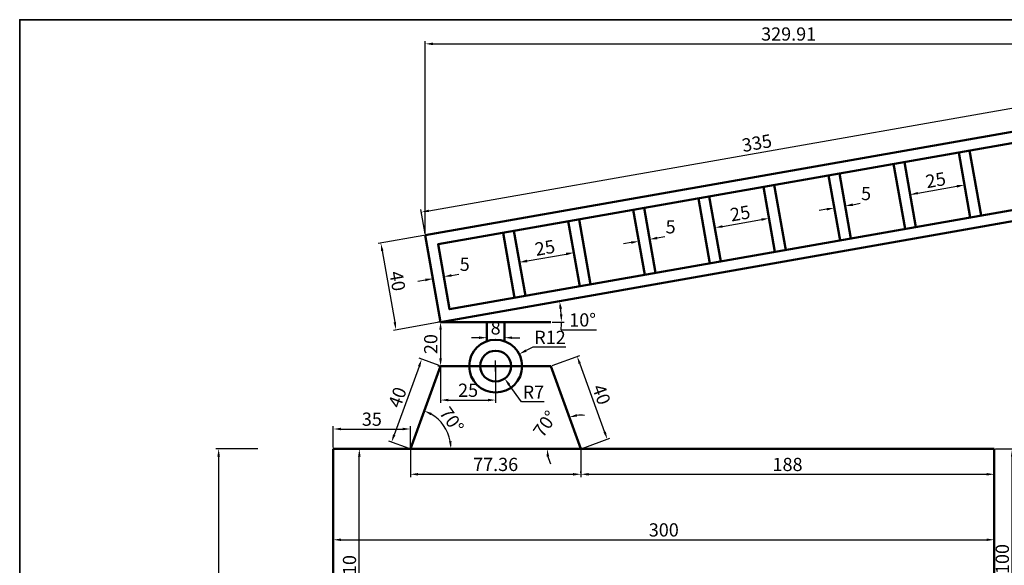
# Model space of a CAD drawing. Units: millimetres. Extents: x -71 to 780, y -41 to 454.
# Tile 2 of 4: x -71 to 376, y 206 to 454. Entities that reach past the tile are written whole.
import ezdxf

# ---------------------------------------------------------------- set-up
doc = ezdxf.new("R2010")
doc.units = ezdxf.units.MM
for name, color, linetype, lineweight in [('M-DIMS', 2, 'Continuous', 25), ('M-OUTL', 7, 'Continuous', 50), ('M-TTLB', 7, 'Continuous', 35)]:
    doc.layers.add(name, color=color, linetype=linetype, lineweight=lineweight)
doc.styles.get("Standard").update_dxf_attribs({"font": 'arial.ttf'})
doc.dimstyles.new('ISO-25', dxfattribs={"dimtxt": 6, "dimasz": 3.5, "dimexe": 1.25, "dimexo": 0.625, "dimtad": 1, "dimtoh": 1, "dimdec": 0, "dimtxsty": 'Standard', "dimcen": 2.5, "dimadec": 0, "dimazin": 0, "dimtfac": 1, "dimtdec": 0, "dimtofl": 0, "dimtmove": 0, "dimatfit": 3, "dimfxl": 1, "dimarcsym": 0})

# ---------------------------------------------------------------- blocks, each defined once
blk = doc.blocks.new('*D10')
at = {"layer": 'Defpoints', "color": 0, "transparency": 16777216}
for p in [(37.81, 259.32), (19.33, 119.32), (37.81, 119.32)]:
    blk.add_point(p, dxfattribs=at)
at = {"layer": 'M-DIMS', "color": 0, "lineweight": -2, "transparency": 16777216}
for p, q in [((37.19, 259.32), (18.08, 259.32)), ((19.33, 255.82), (19.33, 122.82)), ((37.19, 119.32), (18.08, 119.32))]:
    blk.add_line(p, q, dxfattribs=at)
at = {"layer": 'M-DIMS', "color": 0, "transparency": 16777216}
for points in [[(18.74, 255.82), (19.91, 255.82), (19.33, 259.32)], [(18.74, 122.82), (19.91, 122.82), (19.33, 119.32)]]:
    blk.add_solid(points, dxfattribs=at)
at = {"layer": 'M-DIMS', "color": 0, "transparency": 16777216, "insert": (15.64, 189.32), "char_height": 6, "attachment_point": 5, "rotation": 90}
blk.add_mtext('140', dxfattribs=at)
blk = doc.blocks.new('*D11')
at = {"layer": 'Defpoints', "color": 0, "transparency": 16777216}
for p in [(82.72, 259.32), (83.19, 259.32), (82.72, 149.32)]:
    blk.add_point(p, dxfattribs=at)
at = {"layer": 'M-DIMS', "color": 0, "lineweight": -2, "transparency": 16777216}
for p, q in [((83.35, 259.32), (84.44, 259.32)), ((83.19, 152.82), (83.19, 255.82)), ((83.35, 149.32), (84.44, 149.32))]:
    blk.add_line(p, q, dxfattribs=at)
at = {"layer": 'M-DIMS', "color": 0, "transparency": 16777216}
for points in [[(82.61, 255.82), (83.77, 255.82), (83.19, 259.32)], [(82.61, 152.82), (83.77, 152.82), (83.19, 149.32)]]:
    blk.add_solid(points, dxfattribs=at)
at = {"layer": 'M-DIMS', "color": 0, "transparency": 16777216, "insert": (79.5, 204.32), "char_height": 6, "attachment_point": 5, "rotation": 90}
blk.add_mtext('110', dxfattribs=at)
blk = doc.blocks.new('*D13')
at = {"layer": 'Defpoints', "color": 0, "transparency": 16777216}
for p in [(106.38, 268.35), (71.38, 259.32), (106.38, 259.32)]:
    blk.add_point(p, dxfattribs=at)
at = {"layer": 'M-DIMS', "color": 0, "lineweight": -2, "transparency": 16777216}
for p, q in [((71.38, 259.95), (71.38, 269.6)), ((74.88, 268.35), (102.88, 268.35)), ((106.38, 259.95), (106.38, 269.6))]:
    blk.add_line(p, q, dxfattribs=at)
at = {"layer": 'M-DIMS', "color": 0, "transparency": 16777216}
for points in [[(74.88, 268.93), (74.88, 267.77), (71.38, 268.35)], [(102.88, 268.93), (102.88, 267.77), (106.38, 268.35)]]:
    blk.add_solid(points, dxfattribs=at)
at = {"layer": 'M-DIMS', "color": 0, "transparency": 16777216, "insert": (88.88, 272.04), "char_height": 6, "attachment_point": 5}
blk.add_mtext('35', dxfattribs=at)
blk = doc.blocks.new('*D14')
at = {"layer": 'Defpoints', "color": 0, "transparency": 16777216}
for p in [(106.38, 259.32), (183.74, 259.32), (183.74, 247.8)]:
    blk.add_point(p, dxfattribs=at)
at = {"layer": 'M-DIMS', "color": 0, "lineweight": -2, "transparency": 16777216}
for p, q in [((106.38, 258.7), (106.38, 246.55)), ((183.74, 258.7), (183.74, 246.55)), ((109.88, 247.8), (180.24, 247.8))]:
    blk.add_line(p, q, dxfattribs=at)
at = {"layer": 'M-DIMS', "color": 0, "transparency": 16777216}
for points in [[(109.88, 248.38), (109.88, 247.21), (106.38, 247.8)], [(180.24, 248.38), (180.24, 247.21), (183.74, 247.8)]]:
    blk.add_solid(points, dxfattribs=at)
at = {"layer": 'M-DIMS', "color": 0, "transparency": 16777216, "insert": (145.06, 251.49), "char_height": 6, "attachment_point": 5}
blk.add_mtext('77.36', dxfattribs=at)
blk = doc.blocks.new('*D15')
at = {"layer": 'Defpoints', "color": 0, "transparency": 16777216}
for p in [(170.06, 296.91), (195.75, 263.69), (183.74, 259.32)]:
    blk.add_point(p, dxfattribs=at)
at = {"layer": 'M-DIMS', "color": 0, "lineweight": -2, "transparency": 16777216}
for p, q in [((170.65, 297.13), (183.25, 301.71)), ((183.27, 297.99), (194.55, 266.98)), ((184.33, 259.54), (196.93, 264.12))]:
    blk.add_line(p, q, dxfattribs=at)
at = {"layer": 'M-DIMS', "color": 0, "transparency": 16777216}
for points in [[(183.82, 298.19), (182.72, 297.79), (182.07, 301.28)], [(195.1, 267.18), (194.01, 266.78), (195.75, 263.69)]]:
    blk.add_solid(points, dxfattribs=at)
at = {"layer": 'M-DIMS', "color": 0, "transparency": 16777216, "insert": (192.38, 283.75), "char_height": 6, "attachment_point": 5, "rotation": 290}
blk.add_mtext('40', dxfattribs=at)
blk = doc.blocks.new('*D16')
at = {"layer": 'Defpoints', "color": 0, "transparency": 16777216}
for p in [(120.06, 296.91), (97.82, 262.44), (106.38, 259.32)]:
    blk.add_point(p, dxfattribs=at)
at = {"layer": 'M-DIMS', "color": 0, "lineweight": -2, "transparency": 16777216}
for p, q in [((119.48, 297.13), (110.33, 300.46)), ((110.3, 296.74), (99.02, 265.73)), ((105.8, 259.54), (96.65, 262.87))]:
    blk.add_line(p, q, dxfattribs=at)
at = {"layer": 'M-DIMS', "color": 0, "transparency": 16777216}
for points in [[(109.76, 296.94), (110.85, 296.54), (111.5, 300.03)], [(98.47, 265.93), (99.57, 265.53), (97.82, 262.44)]]:
    blk.add_solid(points, dxfattribs=at)
at = {"layer": 'M-DIMS', "color": 0, "transparency": 16777216, "insert": (101.19, 282.5), "char_height": 6, "attachment_point": 5, "rotation": 70}
blk.add_mtext('40', dxfattribs=at)
blk = doc.blocks.new('*D17')
at = {"layer": 'Defpoints', "color": 0, "transparency": 16777216}
for p in [(120.06, 296.91), (123.29, 266.62), (71.38, 259.32), (106.38, 259.32), (371.38, 259.32)]:
    blk.add_point(p, dxfattribs=at)
at = {"layer": 'M-DIMS', "color": 0, "lineweight": -2, "transparency": 16777216}
blk.add_arc((106.38, 259.32), 18.41, 10.9089, 59.0911, dxfattribs=at)
at = {"layer": 'M-DIMS', "color": 0, "transparency": 16777216}
for points in [[(115.59, 274.59), (116.09, 275.65), (112.68, 276.62)], [(125.04, 262.86), (123.88, 262.75), (124.79, 259.32)]]:
    blk.add_solid(points, dxfattribs=at)
at = {"layer": 'M-DIMS', "color": 0, "transparency": 16777216, "insert": (124.49, 272), "char_height": 6, "attachment_point": 5, "rotation": 305}
blk.add_mtext('70°', dxfattribs=at)
blk = doc.blocks.new('*D18')
at = {"layer": 'Defpoints', "color": 0, "transparency": 16777216}
for p in [(170.06, 296.91), (173.23, 270.47), (71.38, 259.32), (183.74, 259.32), (371.38, 259.32)]:
    blk.add_point(p, dxfattribs=at)
at = {"layer": 'M-DIMS', "color": 0, "lineweight": -2, "transparency": 16777216}
for start, end in [(83.7628, 96.8814), (193.1186, 206.2372)]:
    blk.add_arc((183.74, 259.32), 15.32, start, end, dxfattribs=at)
at = {"layer": 'M-DIMS', "color": 0, "transparency": 16777216}
for points in [[(182.04, 273.97), (181.77, 275.1), (178.5, 273.72)], [(168.24, 255.78), (169.4, 255.91), (168.42, 259.32)]]:
    blk.add_solid(points, dxfattribs=at)
at = {"layer": 'M-DIMS', "color": 0, "transparency": 16777216, "insert": (168.17, 270.23), "char_height": 6, "attachment_point": 5, "rotation": 55}
blk.add_mtext('70°', dxfattribs=at)
blk = doc.blocks.new('*D19')
at = {"layer": 'Defpoints', "color": 0, "transparency": 16777216}
for p in [(449.98, 375.08), (174.55, 323.28), (120.06, 316.91), (120.06, 316.91), (170.06, 316.91)]:
    blk.add_point(p, dxfattribs=at)
at = {"layer": 'M-DIMS', "color": 0, "lineweight": -2, "transparency": 16777216}
for p, q in [((170.69, 316.91), (176.17, 316.91)), ((174.81, 313.41), (190.77, 313.41))]:
    blk.add_line(p, q, dxfattribs=at)
for start, end in [(3.6562, 6.3438), (356.3438, 360)]:
    blk.add_arc((120.06, 316.91), 54.86, start, end, dxfattribs=at)
at = {"layer": 'M-DIMS', "color": 0, "transparency": 16777216}
for points in [[(174.01, 322.89), (175.16, 323.06), (174.09, 326.44)], [(175.39, 320.43), (174.23, 320.39), (174.92, 316.91)]]:
    blk.add_solid(points, dxfattribs=at)
at = {"layer": 'M-DIMS', "color": 0, "transparency": 16777216, "insert": (184.54, 317.1), "char_height": 6, "attachment_point": 5}
blk.add_mtext('10°', dxfattribs=at)
blk = doc.blocks.new('*D20')
at = {"layer": 'Defpoints', "color": 0, "transparency": 16777216}
for p in [(113.12, 356.3), (99.89, 313.35), (120.06, 316.91)]:
    blk.add_point(p, dxfattribs=at)
at = {"layer": 'M-DIMS', "color": 0, "lineweight": -2, "transparency": 16777216}
for p, q in [((112.5, 356.2), (91.71, 352.53)), ((93.55, 349.3), (99.28, 316.8)), ((119.45, 316.8), (98.66, 313.14))]:
    blk.add_line(p, q, dxfattribs=at)
at = {"layer": 'M-DIMS', "color": 0, "transparency": 16777216}
for points in [[(94.13, 349.4), (92.98, 349.2), (92.94, 352.75)], [(99.86, 316.9), (98.71, 316.7), (99.89, 313.35)]]:
    blk.add_solid(points, dxfattribs=at)
at = {"layer": 'M-DIMS', "color": 0, "transparency": 16777216, "insert": (99.74, 335.41), "char_height": 6, "attachment_point": 5, "rotation": 280}
blk.add_mtext('40', dxfattribs=at)
blk = doc.blocks.new('*D21')
at = {"layer": 'Defpoints', "color": 0, "transparency": 16777216}
for p in [(441.18, 424.97), (443.03, 414.48), (113.12, 356.3)]:
    blk.add_point(p, dxfattribs=at)
at = {"layer": 'M-DIMS', "color": 0, "lineweight": -2, "transparency": 16777216}
for p, q in [((442.92, 415.09), (440.96, 426.2)), ((114.71, 367.41), (437.73, 424.36)), ((113.01, 356.92), (111.05, 368.03))]:
    blk.add_line(p, q, dxfattribs=at)
at = {"layer": 'M-DIMS', "color": 0, "transparency": 16777216}
for points in [[(437.63, 424.94), (437.83, 423.79), (441.18, 424.97)], [(114.61, 367.98), (114.82, 366.83), (111.27, 366.8)]]:
    blk.add_solid(points, dxfattribs=at)
at = {"layer": 'M-DIMS', "color": 0, "transparency": 16777216, "insert": (263.76, 397.44), "char_height": 6, "attachment_point": 5, "rotation": 10}
blk.add_mtext('335', dxfattribs=at)
blk = doc.blocks.new('*D22')
at = {"layer": 'Defpoints', "color": 0, "transparency": 16777216}
for p in [(116.59, 336.61), (121.52, 337.48), (121.52, 337.48)]:
    blk.add_point(p, dxfattribs=at)
at = {"layer": 'M-DIMS', "color": 0, "lineweight": -2, "transparency": 16777216}
for p, q in [((113.15, 336), (109.7, 335.39)), ((116.7, 335.99), (116.81, 335.38)), ((121.62, 336.86), (121.73, 336.25)), ((124.96, 338.08), (128.41, 338.69))]:
    blk.add_line(p, q, dxfattribs=at)
at = {"layer": 'M-DIMS', "color": 0, "transparency": 16777216}
for points in [[(113.04, 336.57), (113.25, 335.43), (116.59, 336.61)], [(124.86, 338.66), (125.06, 337.51), (121.52, 337.48)]]:
    blk.add_solid(points, dxfattribs=at)
at = {"layer": 'M-DIMS', "color": 0, "transparency": 16777216, "insert": (131.02, 342.37), "char_height": 6, "attachment_point": 5}
blk.add_mtext('5', dxfattribs=at)
blk = doc.blocks.new('*D23')
at = {"layer": 'Defpoints', "color": 0, "transparency": 16777216}
for p in [(180.51, 348.41), (180.6, 347.9), (155.98, 343.55)]:
    blk.add_point(p, dxfattribs=at)
at = {"layer": 'M-DIMS', "color": 0, "lineweight": -2, "transparency": 16777216}
for p, q in [((180.5, 348.51), (180.3, 349.64)), ((155.88, 344.17), (155.68, 345.3)), ((159.34, 344.67), (177.07, 347.8))]:
    blk.add_line(p, q, dxfattribs=at)
at = {"layer": 'M-DIMS', "color": 0, "transparency": 16777216}
for points in [[(159.24, 345.25), (159.44, 344.1), (155.89, 344.07)], [(176.97, 348.37), (177.17, 347.22), (180.51, 348.41)]]:
    blk.add_solid(points, dxfattribs=at)
at = {"layer": 'M-DIMS', "color": 0, "transparency": 16777216, "insert": (167.56, 349.87), "char_height": 6, "attachment_point": 5, "rotation": 10}
blk.add_mtext('25', dxfattribs=at)
blk = doc.blocks.new('*D24')
at = {"layer": 'Defpoints', "color": 0, "transparency": 16777216}
for p in [(210.06, 353.62), (214.98, 354.48), (214.98, 354.48)]:
    blk.add_point(p, dxfattribs=at)
at = {"layer": 'M-DIMS', "color": 0, "lineweight": -2, "transparency": 16777216}
for p, q in [((209.95, 354.23), (209.84, 354.85)), ((214.87, 355.1), (214.77, 355.72)), ((218.43, 355.09), (221.88, 355.7)), ((206.61, 353.01), (203.16, 352.4))]:
    blk.add_line(p, q, dxfattribs=at)
at = {"layer": 'M-DIMS', "color": 0, "transparency": 16777216}
for points in [[(206.51, 353.58), (206.71, 352.43), (210.06, 353.62)], [(218.33, 355.67), (218.53, 354.52), (214.98, 354.48)]]:
    blk.add_solid(points, dxfattribs=at)
at = {"layer": 'M-DIMS', "color": 0, "transparency": 16777216, "insert": (224.49, 359.38), "char_height": 6, "attachment_point": 5}
blk.add_mtext('5', dxfattribs=at)
blk = doc.blocks.new('*D25')
at = {"layer": 'Defpoints', "color": 0, "transparency": 16777216}
for p in [(269.15, 364.03), (269.15, 364.03), (244.53, 359.69)]:
    blk.add_point(p, dxfattribs=at)
at = {"layer": 'M-DIMS', "color": 0, "lineweight": -2, "transparency": 16777216}
for p, q in [((247.97, 360.3), (265.7, 363.43)), ((269.26, 363.42), (269.36, 362.8)), ((244.64, 359.08), (244.74, 358.46))]:
    blk.add_line(p, q, dxfattribs=at)
at = {"layer": 'M-DIMS', "color": 0, "transparency": 16777216}
for points in [[(265.6, 364), (265.8, 362.85), (269.15, 364.03)], [(247.87, 360.88), (248.07, 359.73), (244.53, 359.69)]]:
    blk.add_solid(points, dxfattribs=at)
at = {"layer": 'M-DIMS', "color": 0, "transparency": 16777216, "insert": (256.2, 365.5), "char_height": 6, "attachment_point": 5, "rotation": 10}
blk.add_mtext('25', dxfattribs=at)
blk = doc.blocks.new('*D26')
at = {"layer": 'Defpoints', "color": 0, "transparency": 16777216}
for p in [(298.78, 368.73), (303.71, 369.6), (303.71, 369.6)]:
    blk.add_point(p, dxfattribs=at)
at = {"layer": 'M-DIMS', "color": 0, "lineweight": -2, "transparency": 16777216}
for p, q in [((295.33, 368.13), (291.89, 367.52)), ((298.67, 369.35), (298.56, 369.96)), ((303.6, 370.22), (303.49, 370.83)), ((307.15, 370.21), (310.6, 370.82))]:
    blk.add_line(p, q, dxfattribs=at)
at = {"layer": 'M-DIMS', "color": 0, "transparency": 16777216}
for points in [[(295.23, 368.7), (295.44, 367.55), (298.78, 368.73)], [(307.05, 370.78), (307.25, 369.63), (303.71, 369.6)]]:
    blk.add_solid(points, dxfattribs=at)
at = {"layer": 'M-DIMS', "color": 0, "transparency": 16777216, "insert": (313.21, 374.49), "char_height": 6, "attachment_point": 5}
blk.add_mtext('5', dxfattribs=at)
blk = doc.blocks.new('*D27')
at = {"layer": 'Defpoints', "color": 0, "transparency": 16777216}
for p in [(357.87, 379.15), (357.87, 379.15), (333.25, 374.81)]:
    blk.add_point(p, dxfattribs=at)
at = {"layer": 'M-DIMS', "color": 0, "lineweight": -2, "transparency": 16777216}
for p, q in [((357.76, 379.77), (357.65, 380.38)), ((336.7, 375.42), (354.42, 378.54)), ((333.36, 374.19), (333.47, 373.58))]:
    blk.add_line(p, q, dxfattribs=at)
at = {"layer": 'M-DIMS', "color": 0, "transparency": 16777216}
for points in [[(336.6, 375.99), (336.8, 374.84), (333.25, 374.81)], [(354.32, 379.12), (354.52, 377.97), (357.87, 379.15)]]:
    blk.add_solid(points, dxfattribs=at)
at = {"layer": 'M-DIMS', "color": 0, "transparency": 16777216, "insert": (344.92, 380.61), "char_height": 6, "attachment_point": 5, "rotation": 10}
blk.add_mtext('25', dxfattribs=at)
blk = doc.blocks.new('*D31')
at = {"layer": 'Defpoints', "color": 0, "transparency": 16777216}
for p in [(71.38, 225.97), (371.38, 225.97), (371.38, 218.07)]:
    blk.add_point(p, dxfattribs=at)
at = {"layer": 'M-DIMS', "color": 0, "lineweight": -2, "transparency": 16777216}
for p, q in [((71.38, 225.35), (71.38, 216.82)), ((371.38, 225.35), (371.38, 216.82)), ((74.88, 218.07), (367.88, 218.07))]:
    blk.add_line(p, q, dxfattribs=at)
at = {"layer": 'M-DIMS', "color": 0, "transparency": 16777216}
for points in [[(74.88, 218.65), (74.88, 217.49), (71.38, 218.07)], [(367.88, 218.65), (367.88, 217.49), (371.38, 218.07)]]:
    blk.add_solid(points, dxfattribs=at)
at = {"layer": 'M-DIMS', "color": 0, "transparency": 16777216, "insert": (221.38, 221.76), "char_height": 6, "attachment_point": 5}
blk.add_mtext('300', dxfattribs=at)
blk = doc.blocks.new('*D32')
at = {"layer": 'Defpoints', "color": 0, "transparency": 16777216}
for p in [(183.74, 247.8), (371.38, 247.8), (371.38, 247.8)]:
    blk.add_point(p, dxfattribs=at)
at = {"layer": 'M-DIMS', "color": 0, "lineweight": -2, "transparency": 16777216}
for p, q in [((183.74, 248.42), (183.74, 249.05)), ((187.24, 247.8), (367.88, 247.8)), ((371.38, 248.42), (371.38, 249.05))]:
    blk.add_line(p, q, dxfattribs=at)
at = {"layer": 'M-DIMS', "color": 0, "transparency": 16777216}
for points in [[(187.24, 248.38), (187.24, 247.21), (183.74, 247.8)], [(367.88, 248.38), (367.88, 247.21), (371.38, 247.8)]]:
    blk.add_solid(points, dxfattribs=at)
at = {"layer": 'M-DIMS', "color": 0, "transparency": 16777216, "insert": (277.56, 251.48), "char_height": 6, "attachment_point": 5}
blk.add_mtext('188', dxfattribs=at)
blk = doc.blocks.new('*D75')
at = {"layer": 'Defpoints', "color": 0, "transparency": 16777216}
for p in [(371.38, 259.32), (379.51, 259.32), (371.38, 159.32)]:
    blk.add_point(p, dxfattribs=at)
at = {"layer": 'M-DIMS', "color": 0, "lineweight": -2, "transparency": 16777216}
for p, q in [((372.01, 259.32), (380.76, 259.32)), ((379.51, 162.82), (379.51, 255.82)), ((372.01, 159.32), (380.76, 159.32))]:
    blk.add_line(p, q, dxfattribs=at)
at = {"layer": 'M-DIMS', "color": 0, "transparency": 16777216}
for points in [[(378.92, 255.82), (380.09, 255.82), (379.51, 259.32)], [(378.92, 162.82), (380.09, 162.82), (379.51, 159.32)]]:
    blk.add_solid(points, dxfattribs=at)
at = {"layer": 'M-DIMS', "color": 0, "transparency": 16777216, "insert": (375.82, 209.32), "char_height": 6, "attachment_point": 5, "rotation": 90}
blk.add_mtext('100', dxfattribs=at)
blk = doc.blocks.new('*D77')
at = {"layer": 'Defpoints', "color": 0, "transparency": 16777216}
for p in [(155.75, 302.38), (145.06, 296.91)]:
    blk.add_point(p, dxfattribs=at)
at = {"layer": 'M-DIMS', "color": 0, "lineweight": -2, "transparency": 16777216}
for p, q in [((161.98, 305.56), (158.86, 303.97)), ((176.88, 305.56), (161.98, 305.56)), ((142.56, 296.91), (147.56, 296.91)), ((145.06, 294.41), (145.06, 299.41))]:
    blk.add_line(p, q, dxfattribs=at)
at = {"layer": 'M-DIMS', "color": 0, "transparency": 16777216}
blk.add_solid([(158.6, 304.49), (159.13, 303.45), (155.75, 302.38)], dxfattribs=at)
at = {"layer": 'M-DIMS', "color": 0, "transparency": 16777216, "insert": (169.74, 309.2), "char_height": 6, "attachment_point": 5}
blk.add_mtext('R12', dxfattribs=at)
blk = doc.blocks.new('*D78')
at = {"layer": 'Defpoints', "color": 0, "transparency": 16777216}
for p in [(145.06, 296.91), (149.15, 291.23)]:
    blk.add_point(p, dxfattribs=at)
at = {"layer": 'M-DIMS', "color": 0, "lineweight": -2, "transparency": 16777216}
for p, q in [((142.56, 296.91), (147.56, 296.91)), ((145.06, 294.41), (145.06, 299.41)), ((156.75, 280.68), (151.2, 288.39)), ((167.05, 280.68), (156.75, 280.68))]:
    blk.add_line(p, q, dxfattribs=at)
at = {"layer": 'M-DIMS', "color": 0, "transparency": 16777216}
blk.add_solid([(151.67, 288.73), (150.73, 288.05), (149.15, 291.23)], dxfattribs=at)
at = {"layer": 'M-DIMS', "color": 0, "transparency": 16777216, "insert": (162.21, 284.31), "char_height": 6, "attachment_point": 5}
blk.add_mtext('R7', dxfattribs=at)
blk = doc.blocks.new('*D79')
at = {"layer": 'Defpoints', "color": 0, "transparency": 16777216}
for p in [(141.06, 316.91), (149.06, 316.91), (149.06, 309.81)]:
    blk.add_point(p, dxfattribs=at)
at = {"layer": 'M-DIMS', "color": 0, "lineweight": -2, "transparency": 16777216}
for p, q in [((141.06, 316.29), (141.06, 308.56)), ((149.06, 316.29), (149.06, 308.56)), ((137.56, 309.81), (134.06, 309.81)), ((152.56, 309.81), (156.06, 309.81))]:
    blk.add_line(p, q, dxfattribs=at)
at = {"layer": 'M-DIMS', "color": 0, "transparency": 16777216}
for points in [[(137.56, 310.39), (137.56, 309.22), (141.06, 309.81)], [(152.56, 310.39), (152.56, 309.22), (149.06, 309.81)]]:
    blk.add_solid(points, dxfattribs=at)
at = {"layer": 'M-DIMS', "color": 0, "transparency": 16777216, "insert": (145.06, 313.49), "char_height": 6, "attachment_point": 5}
blk.add_mtext('8', dxfattribs=at)
blk = doc.blocks.new('*D80')
at = {"layer": 'Defpoints', "color": 0, "transparency": 16777216}
for p in [(124.07, 316.91), (120.06, 296.91), (124.07, 296.91)]:
    blk.add_point(p, dxfattribs=at)
at = {"layer": 'M-DIMS', "color": 0, "lineweight": -2, "transparency": 16777216}
for p, q in [((123.44, 316.91), (118.81, 316.91)), ((120.06, 313.41), (120.06, 300.41)), ((123.44, 296.91), (118.81, 296.91))]:
    blk.add_line(p, q, dxfattribs=at)
at = {"layer": 'M-DIMS', "color": 0, "transparency": 16777216}
for points in [[(119.48, 313.41), (120.65, 313.41), (120.06, 316.91)], [(119.48, 300.41), (120.65, 300.41), (120.06, 296.91)]]:
    blk.add_solid(points, dxfattribs=at)
at = {"layer": 'M-DIMS', "color": 0, "transparency": 16777216, "insert": (116.38, 306.91), "char_height": 6, "attachment_point": 5, "rotation": 90}
blk.add_mtext('20', dxfattribs=at)
blk = doc.blocks.new('*D81')
at = {"layer": 'Defpoints', "color": 0, "transparency": 16777216}
for p in [(120.06, 296.91), (145.06, 296.91), (145.06, 281.5)]:
    blk.add_point(p, dxfattribs=at)
at = {"layer": 'M-DIMS', "color": 0, "lineweight": -2, "transparency": 16777216}
for p, q in [((120.06, 296.29), (120.06, 280.25)), ((145.06, 296.29), (145.06, 280.25)), ((123.56, 281.5), (141.56, 281.5))]:
    blk.add_line(p, q, dxfattribs=at)
at = {"layer": 'M-DIMS', "color": 0, "transparency": 16777216}
for points in [[(123.56, 282.08), (123.56, 280.91), (120.06, 281.5)], [(141.56, 282.08), (141.56, 280.91), (145.06, 281.5)]]:
    blk.add_solid(points, dxfattribs=at)
at = {"layer": 'M-DIMS', "color": 0, "transparency": 16777216, "insert": (132.56, 285.18), "char_height": 6, "attachment_point": 5}
blk.add_mtext('25', dxfattribs=at)
blk = doc.blocks.new('*D84')
at = {"layer": 'Defpoints', "color": 0, "transparency": 16777216}
for p in [(443.03, 443.23), (443.03, 414.48), (113.12, 356.3)]:
    blk.add_point(p, dxfattribs=at)
at = {"layer": 'M-DIMS', "color": 0, "lineweight": -2, "transparency": 16777216}
for p, q in [((113.12, 356.93), (113.12, 444.48)), ((116.62, 443.23), (439.53, 443.23)), ((443.03, 415.1), (443.03, 444.48))]:
    blk.add_line(p, q, dxfattribs=at)
at = {"layer": 'M-DIMS', "color": 0, "transparency": 16777216}
for points in [[(116.62, 443.81), (116.62, 442.64), (113.12, 443.23)], [(439.53, 443.81), (439.53, 442.64), (443.03, 443.23)]]:
    blk.add_solid(points, dxfattribs=at)
at = {"layer": 'M-DIMS', "color": 0, "transparency": 16777216, "insert": (278.07, 446.92), "char_height": 6, "attachment_point": 5}
blk.add_mtext('329.91', dxfattribs=at)

msp = doc.modelspace()

# ---------------------------------------------------------------- linework, layer by layer
at = {"layer": 'M-OUTL'}
for p, q in [((355.265, 393.924), (360.475, 364.38)), ((360.189, 394.792), (365.399, 365.248)), ((330.645, 389.583), (335.854, 360.038)), ((301.101, 384.373), (306.31, 354.829)), ((325.721, 388.714), (330.93, 359.17)), ((296.177, 383.505), (301.386, 353.961)), ((266.632, 378.295), (271.842, 348.751)), ((271.556, 379.164), (276.766, 349.619)), ((237.088, 373.086), (242.298, 343.542)), ((242.012, 373.954), (247.222, 344.41)), ((207.544, 367.877), (212.753, 338.332)), ((212.468, 368.745), (217.677, 339.201)), ((178, 362.667), (183.209, 333.123)), ((182.924, 363.535), (188.133, 333.991)), ((153.379, 358.326), (158.589, 328.782)), ((148.455, 357.458), (153.665, 327.913)), ((118.911, 352.248), (124.121, 322.704)), ((170.063, 316.912), (120.065, 316.912)), ((141.064, 308.225), (141.064, 316.912)), ((149.064, 308.225), (149.064, 316.912)), ((106.384, 259.324), (120.065, 296.912)), ((170.063, 296.912), (120.065, 296.912)), ((183.744, 259.324), (170.063, 296.912)), ((71.384, 124.324), (71.384, 259.324)), ((71.384, 259.324), (371.384, 259.324)), ((371.384, 259.324), (371.384, 159.324))]:
    msp.add_line(p, q, dxfattribs=at)
for points in [[(449.975, 375.084), (120.065, 316.912), (113.119, 356.304), (443.03, 414.476, -1)], [(449.107, 380.008), (124.121, 322.704), (118.911, 352.248), (443.898, 409.552, -1)]]:
    msp.add_lwpolyline(points, format="xyb", close=True, dxfattribs=at)
for radius in [12, 7]:
    msp.add_circle((145.064, 296.912), radius, dxfattribs=at)
at = {"layer": 'M-TTLB'}
msp.add_lwpolyline([(779.526, -41.268), (-70.976, -41.268), (-70.976, 454.198), (779.526, 454.198)], close=True, dxfattribs=at)

# ---------------------------------------------------------------- dimensions: what is measured, and where the dimension line sits
at = {"layer": 'M-DIMS'}
for base, p1, p2, override, picture, middle in [((443.03, 443.226), (113.119, 356.304), (443.03, 414.476), {"dimdec": 2, "dimlfac": 1, "dimrnd": 0, "dimzin": 0, "dimdsep": 46, "dimlunit": 2}, '*D84', (278.074, 446.917)), ((149.064, 309.806), (141.064, 316.912), (149.064, 316.912), {"dimclrd": 0, "dimclre": 0, "dimclrt": 0}, '*D79', (145.064, 313.495)), ((145.064, 281.496), (120.065, 296.912), (145.064, 296.912), {"dimclrd": 0, "dimclre": 0, "dimclrt": 0}, '*D81', (132.564, 285.184)), ((106.384, 268.351), (71.384, 259.324), (106.384, 259.324), {"dimclrd": 0, "dimclre": 0, "dimclrt": 0}, '*D13', (88.884, 272.042)), ((371.384, 247.796), (183.744, 247.796), (371.384, 247.796), {"dimclrd": 0, "dimclre": 0, "dimclrt": 0}, '*D32', (277.564, 251.484)), ((371.384, 218.072), (71.384, 225.97), (371.384, 225.97), {"dimclrd": 0, "dimclre": 0, "dimclrt": 0}, '*D31', (221.384, 221.762))]:
    dim = msp.add_linear_dim(base=base, p1=p1, p2=p2, dimstyle='ISO-25', override=override, dxfattribs=at)
    dim.commit()
    dim.dimension.update_dxf_attribs({"geometry": picture, "text_midpoint": middle})
for base, p2, angle, picture, middle in [((441.179, 424.973), (443.03, 414.476), 10, '*D21', (264.402, 393.802)), ((99.889, 313.354), (120.065, 316.912), 280, '*D20', (96.112, 334.772))]:
    dim = msp.add_linear_dim(base=base, p1=(113.119, 356.304), p2=p2, angle=angle, dimstyle='ISO-25', override={"dimclrd": 0, "dimclre": 0, "dimclrt": 0}, dxfattribs=at)
    dim.commit()
    dim.dimension.update_dxf_attribs({"geometry": picture, "text_midpoint": middle, "dimtype": 161})
for p1, p2, distance, picture, middle in [((333.25, 374.811), (357.87, 379.152), 0, '*D27', (344.919, 380.614)), ((298.781, 368.733), (303.705, 369.601), 0, '*D26', (313.213, 374.493)), ((244.527, 359.694), (269.147, 364.035), 0, '*D25', (256.196, 365.497)), ((210.058, 353.616), (214.982, 354.484), 0, '*D24', (224.49, 359.376)), ((155.984, 343.554), (180.604, 347.895), 0.52, '*D23', (167.564, 349.868)), ((116.592, 336.608), (121.516, 337.476), 0, '*D22', (131.024, 342.368)), ((120.065, 296.912), (106.384, 259.324), -9.113, '*D16', (101.195, 282.496)), ((170.063, 296.912), (183.744, 259.324), 12.778, '*D15', (192.377, 283.75))]:
    dim = msp.add_aligned_dim(p1=p1, p2=p2, distance=distance, dimstyle='ISO-25', override={"dimclrd": 0, "dimclre": 0, "dimclrt": 0}, dxfattribs=at)
    dim.commit()
    dim.dimension.update_dxf_attribs({"geometry": picture, "text_midpoint": middle})
for base, line1, line2, picture, middle in [((174.551, 323.28), ((170.063, 316.912), (120.065, 316.912)), ((449.975, 375.084), (120.065, 316.912)), '*D19', (184.539, 317.102)), ((123.289, 266.616), ((71.384, 259.324), (371.384, 259.324)), ((106.384, 259.324), (120.065, 296.912)), '*D17', (124.486, 271.999)), ((173.231, 270.467), ((71.384, 259.324), (371.384, 259.324)), ((183.744, 259.324), (170.063, 296.912)), '*D18', (168.173, 270.227))]:
    dim = msp.add_angular_dim_2l(base=base, line1=line1, line2=line2, dimstyle='ISO-25', override={"dimclrd": 0, "dimclre": 0, "dimclrt": 0}, dxfattribs=at)
    dim.commit()
    dim.dimension.update_dxf_attribs({"geometry": picture, "text_midpoint": middle})
for base, p1, p2, picture, middle in [((120.065, 296.912), (124.069, 316.912), (124.069, 296.912), '*D80', (116.376, 306.912)), ((19.328, 119.324), (37.815, 259.324), (37.815, 119.324), '*D10', (15.639, 189.324)), ((83.19, 259.324), (82.724, 149.324), (82.724, 259.324), '*D11', (79.501, 204.324)), ((379.507, 259.324), (371.384, 159.324), (371.384, 259.324), '*D75', (375.819, 209.324))]:
    dim = msp.add_linear_dim(base=base, p1=p1, p2=p2, angle=90, dimstyle='ISO-25', override={"dimclrd": 0, "dimclre": 0, "dimclrt": 0}, dxfattribs=at)
    dim.commit()
    dim.dimension.update_dxf_attribs({"geometry": picture, "text_midpoint": middle})
for mpoint, picture, middle in [((155.748, 302.376), '*D77', (169.742, 309.201)), ((149.155, 291.231), '*D78', (162.214, 284.307))]:
    dim = msp.add_radius_dim(center=(145.064, 296.912), mpoint=mpoint, dimstyle='ISO-25', override={"dimclrd": 0, "dimclre": 0, "dimclrt": 0}, dxfattribs=at)
    dim.commit()
    dim.dimension.update_dxf_attribs({"geometry": picture, "text_midpoint": middle})
dim = msp.add_linear_dim(base=(183.744, 247.796), p1=(106.384, 259.324), p2=(183.744, 259.324), text='<>.36', dimstyle='ISO-25', override={"dimclrd": 0, "dimclre": 0, "dimclrt": 0}, dxfattribs=at)
dim.commit()
dim.dimension.update_dxf_attribs({"geometry": '*D14', "text_midpoint": (145.064, 251.486)})

doc.saveas('drawing.dxf')
